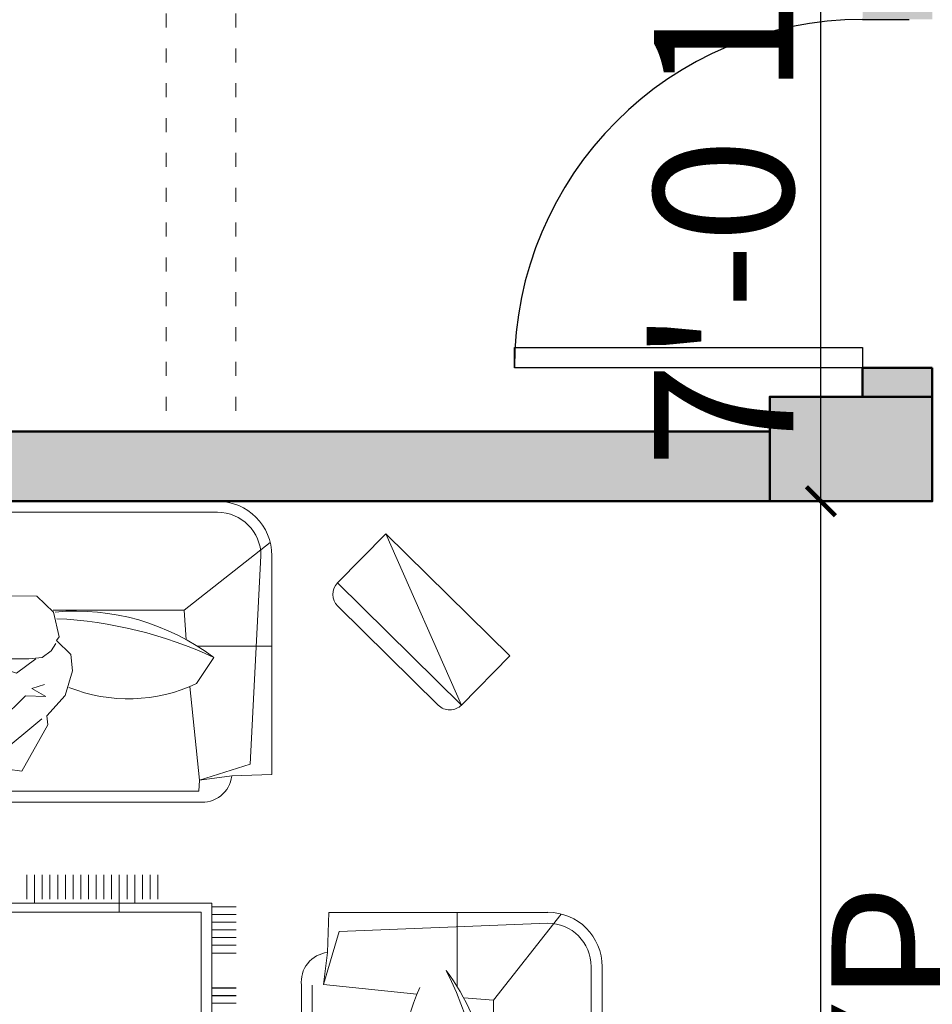
# Model space of a CAD drawing. Units: inches. Extents: x 375 to 1122, y 27 to 1069.
# Tile 76 of 155: x 588 to 667, y 792 to 877. Entities that reach past the tile are written whole.
import ezdxf

# ---------------------------------------------------------------- set-up
doc = ezdxf.new("R2010")
doc.units = ezdxf.units.IN
doc.linetypes.add('ACAD_ISO03W100', pattern=[30, 12, -18])
for name, color, linetype, lineweight in [('A-ANNO-DIMS', 2, 'Continuous', 18), ('A-COLS-PATT', 10, 'Continuous', 13), ('A-WALL-OVHD', 77, 'ACAD_ISO03W100', 18), ('A-WALL-PATT', 252, 'Continuous', 13), ('Columns', 10, 'Continuous', 50), ('Doors', 150, 'Continuous', 25), ('Furniture', 30, 'Continuous', 18), ('Walls', 250, 'Continuous', 50)]:
    doc.layers.add(name, color=color, linetype=linetype, lineweight=lineweight)
doc.styles.get("Standard").update_dxf_attribs({"font": 'arial.ttf'})
doc.dimstyles.new('ISO-25', dxfattribs={"dimtxt": 12, "dimasz": 2.5, "dimexe": 1.5, "dimexo": 1.5, "dimtad": 1, "dimdec": 1, "dimlunit": 3, "dimtxsty": 'Standard', "dimblk": 'ARCHTICK', "dimcen": 2.5, "dimadec": 0, "dimazin": 0, "dimtfac": 1, "dimtdec": 1, "dimtmove": 0, "dimatfit": 3, "dimfxl": 1.5, "dimfxlon": 1, "dimarcsym": 0})

# ---------------------------------------------------------------- blocks, each defined once
blk = doc.blocks.new('*U10')
for p, q in [((-30, 0), (-30, 4)), ((0, 0), (0, 4))]:
    blk.add_line(p, q)
blk.add_lwpolyline([(0, 0), (0, -30), (-1.75, -30), (-1.75, 0)], close=True)
blk.add_arc((0, 0), 30, 180, 270)
blk = doc.blocks.new('A$C4DC51D13')
for p, q in [((3265.3, 2996.2), (1188.4, 2996.2)), ((3265.3, 2962.7), (2590.4, 2962.7)), ((3778.5, 2897), (3631.2, 2747.3)), ((4008.9, 2375.5), (3778.5, 2897)), ((4156.2, 2525.2), (3778.5, 2897)), ((3163.3, 2664.8), (3425.7, 2870.9)), ((3397.7, 2830.3), (3364.5, 2194.8)), ((3430.8, 2163.8), (3430.8, 2830.3)), ((4008.9, 2375.5), (3631.2, 2747.3)), ((3631.7, 2676.6), (3938.2, 2375)), ((3163.3, 2664.8), (2764.7, 2664.8)), ((3170.4, 2574.2), (3163.3, 2664.8)), ((3430.8, 2554.4), (3204.1, 2554.4)), ((3253.7, 2520.5), (3201.8, 2440.8)), ((4008.9, 2375.5), (4156.2, 2525.2)), ((3210.5, 2146.7), (3181.5, 2431.8)), ((3364.5, 2194.8), (3210.5, 2146.7)), ((3308.6, 2159.3), (3430.8, 2163.8)), ((3208.9, 2113), (3210.5, 2146.7)), ((3308.6, 2159.3), (3210.5, 2146.7)), ((2614.2, 2113), (3208.9, 2113)), ((2614.2, 2079.9), (3208.9, 2079.9)), ((2684.5, 1784.3), (2684.5, 1858.2)), ((2708, 1772.3), (2708, 1858.2)), ((2731.5, 1784.3), (2731.5, 1858.2)), ((2754.9, 1784.3), (2754.9, 1858.2)), ((2778.4, 1784.3), (2778.4, 1858.2)), ((2801.9, 1784.3), (2801.9, 1858.2)), ((2825.4, 1784.3), (2825.4, 1858.2)), ((2848.8, 1784.3), (2848.8, 1858.2)), ((2872.3, 1784.3), (2872.3, 1858.2)), ((2895.8, 1784.3), (2895.8, 1858.2)), ((2919.3, 1784.3), (2919.3, 1858.2)), ((2942.7, 1784.3), (2942.7, 1858.2)), ((2966.2, 1744.8), (2966.2, 1858.2)), ((2989.7, 1784.3), (2989.7, 1858.2)), ((3013.2, 1772.3), (3013.2, 1858.2)), ((3036.6, 1784.3), (3036.6, 1858.2)), ((3060.1, 1784.3), (3060.1, 1858.2)), ((3083.6, 1784.3), (3083.6, 1858.2)), ((3248.4, 1772.3), (1158.5, 1772.3)), ((3248.4, 487.7), (3248.4, 1772.3)), ((1196, 1744.8), (3215.6, 1744.8)), ((3215.6, 511), (3215.6, 1744.8)), ((3248.8, 1760.8), (3322.7, 1760.8)), ((3600.6, 1621.7), (3605.1, 1743.8)), ((3605.1, 1743.8), (4271.6, 1743.8)), ((3995.7, 1743.8), (3995.7, 1517.1)), ((3248.8, 1737.3), (3322.7, 1737.3)), ((3248.8, 1713.8), (3322.7, 1713.8)), ((4271.6, 1710.7), (3636.1, 1685.8)), ((4106.1, 1476.4), (4312.2, 1738.8)), ((3248.8, 1690.4), (3322.7, 1690.4)), ((3636.1, 1685.8), (3588, 1523.6)), ((3248.8, 1666.9), (3322.7, 1666.9)), ((3248.8, 1643.4), (3322.7, 1643.4)), ((3248.8, 1619.9), (3322.7, 1619.9)), ((3600.6, 1621.7), (3588, 1523.6)), ((4404, 1578.3), (4404, 904.6)), ((4437.5, 165.9), (4437.5, 1578.3)), ((3248.8, 1513.8), (3322.7, 1513.8)), ((3248.8, 1513.3), (3322.7, 1513.3)), ((3521.2, 1130.7), (3521.2, 1521.9)), ((3554.3, 1131.4), (3554.3, 1521.9)), ((3588, 1523.6), (3873.1, 1494.5)), ((3248.8, 1490.4), (3322.7, 1490.4)), ((3248.8, 1489.9), (3322.7, 1489.9)), ((4015.5, 1483.4), (4106.1, 1476.4)), ((4106.1, 1476.4), (4106.1, 872.1)), ((3248.8, 1466.9), (3322.7, 1466.9))]:
    blk.add_line(p, q)
at = {"linetype": 'ByBlock'}
for points in [[(2625.9, 2180.3), (2669, 2174.2), (2748.1, 2315.4), (2745.8, 2342.6), (2801.2, 2404.9), (2823.9, 2479.6), (2818.4, 2529.9), (2775.1, 2571.7), (2782.4, 2583.3), (2765.2, 2658.8), (2714.5, 2706.9), (2634.6, 2708.6)], [(2563.4, 2654.7), (2512.2, 2609.3), (2506.2, 2548.3), (2540.1, 2504.4), (2576.9, 2490.9), (2579.8, 2539.3), (2598.7, 2543.6), (2636.7, 2516.4), (2690.3, 2516.7), (2731.2, 2520.1), (2758.5, 2540.1), (2773, 2563.3)], [(2712.3, 2515.8), (2652.7, 2472.4), (2603.2, 2489), (2580, 2503.6)], [(2738, 2438.2), (2699.2, 2425.4), (2742.4, 2401.4), (2680.4, 2403.2), (2604.1, 2328.3), (2519.2, 2273.3), (2529.8, 2261.8), (2402.7, 2252.7), (2395.4, 2241.1), (2431.1, 2241.3), (2375.7, 2196.9), (2385.2, 2181.2), (2474.4, 2199.5), (2549.9, 2234.6), (2596.2, 2223.2), (2730.1, 2333.1)]]:
    blk.add_lwpolyline(points, dxfattribs=at)
for centre, radius, start, end in [((3265.3, 2830.3), 165.9, 0, 90), ((3265.3, 2830.3), 132.4, 0, 90), ((3666.8, 2712.2), 50, 135.4503, 225.4503), ((2832.8, 1963.1), 698.5, 52.9389, 95.0789), ((2713.3, 1357.7), 1282.3, 65.0725, 87.2152), ((2993.8, 2882.7), 488.4, 248.2152, 295.2134), ((3973.2, 2410.6), 50, 225.4503, 315.4503), ((3219.2, 2169.3), 90, 263.4179, 353.5749), ((4271.6, 1578.3), 165.9, 0, 90), ((4271.6, 1578.3), 132.4, 0, 90), ((3610.6, 1532.2), 90, 96.4251, 186.5821), ((3383, 1136.2), 721.4, 348.1046, 36.6442), ((2968.3, 1058.8), 1115.8, 356.7543, 27.0804), ((4324, 1306.8), 488.4, 154.7866, 202.7137)]:
    blk.add_arc(centre, radius, start, end)
blk = doc.blocks.new('COLUMN-14X9IN')
blk.add_lwpolyline([(0, 0), (14, 0), (14, 9), (0, 9)], close=True)
blk = doc.blocks.new('_ArchTick')
at = {"color": 0, "linetype": 'ByBlock', "const_width": 0.15}
blk.add_lwpolyline([(-0.5, -0.5), (0.5, 0.5)], dxfattribs=at)
blk = doc.blocks.new('*D58')
at = {"layer": 'A-ANNO-DIMS', "color": 0, "lineweight": -2, "transparency": 16777216}
for p, q in [((656.912, 835.528), (656.912, 940.287)), ((655.412, 835.528), (658.412, 835.528)), ((656.912, 750.836), (656.912, 835.528)), ((655.412, 750.836), (658.412, 750.836))]:
    blk.add_line(p, q, dxfattribs=at)
at = {"layer": 'Defpoints', "color": 0, "transparency": 16777216}
for p in [(638.071, 835.528), (656.912, 835.528), (638.071, 750.836)]:
    blk.add_point(p, dxfattribs=at)
at = {"layer": 'A-ANNO-DIMS', "color": 0, "lineweight": -2, "transparency": 16777216, "xscale": 2.5, "yscale": 2.5, "zscale": 2.5}
for p, rotation in [((656.912, 835.528), 90), ((656.912, 750.836), 270)]:
    blk.add_blockref('_ArchTick', p, dxfattribs=dict(at, rotation=rotation))
at = {"layer": 'A-ANNO-DIMS', "color": 0, "transparency": 16777216, "insert": (650.082, 889.157), "char_height": 12, "attachment_point": 5, "rotation": 90}
blk.add_mtext('7\'-0 1/2" TYP.', dxfattribs=at)
blk = doc.blocks.new('*D79')
at = {"layer": 'A-ANNO-DIMS', "color": 0, "lineweight": -2, "transparency": 16777216}
for p, q in [((672.207, 647.528), (672.207, 810.92)), ((670.707, 647.528), (673.707, 647.528)), ((672.207, 589.528), (672.207, 647.528)), ((670.707, 589.528), (673.707, 589.528))]:
    blk.add_line(p, q, dxfattribs=at)
at = {"layer": 'Defpoints', "color": 0, "transparency": 16777216}
for p in [(663.507, 647.528), (672.207, 647.528), (663.507, 589.528)]:
    blk.add_point(p, dxfattribs=at)
at = {"layer": 'A-ANNO-DIMS', "color": 0, "lineweight": -2, "transparency": 16777216, "xscale": 2.5, "yscale": 2.5, "zscale": 2.5}
for p, rotation in [((672.207, 647.528), 90), ((672.207, 589.528), 270)]:
    blk.add_blockref('_ArchTick', p, dxfattribs=dict(at, rotation=rotation))
at = {"layer": 'A-ANNO-DIMS', "color": 0, "transparency": 16777216, "insert": (665.378, 730.474), "char_height": 12, "attachment_point": 5, "rotation": 90}
blk.add_mtext('CABINET 4\'-10" TYP.', dxfattribs=at)
blk = doc.blocks.new('*D82')
at = {"layer": 'A-ANNO-DIMS', "color": 0, "lineweight": -2, "transparency": 16777216}
for p, q in [((401.507, 1009.528), (398.507, 1009.528)), ((400.007, 160.528), (400.007, 1009.528)), ((401.507, 160.528), (398.507, 160.528))]:
    blk.add_line(p, q, dxfattribs=at)
at = {"layer": 'Defpoints', "color": 0, "transparency": 16777216}
for p in [(400.007, 1009.528), (630.534, 1009.528), (630.534, 160.528)]:
    blk.add_point(p, dxfattribs=at)
at = {"layer": 'A-ANNO-DIMS', "color": 0, "lineweight": -2, "transparency": 16777216, "xscale": 2.5, "yscale": 2.5, "zscale": 2.5}
for p, rotation in [((400.007, 1009.528), 90), ((400.007, 160.528), 270)]:
    blk.add_blockref('_ArchTick', p, dxfattribs=dict(at, rotation=rotation))
at = {"layer": 'A-ANNO-DIMS', "color": 0, "transparency": 16777216, "insert": (393.255, 585.028), "char_height": 12, "attachment_point": 5, "rotation": 90}
blk.add_mtext('70\'-9"', dxfattribs=at)
blk = doc.blocks.new('*D85')
at = {"layer": 'A-ANNO-DIMS', "color": 0, "lineweight": -2, "transparency": 16777216}
for p, q in [((401.507, 868.528), (398.507, 868.528)), ((400.007, 814.528), (400.007, 868.528)), ((401.507, 814.528), (398.507, 814.528))]:
    blk.add_line(p, q, dxfattribs=at)
at = {"layer": 'Defpoints', "color": 0, "transparency": 16777216}
for p in [(400.007, 868.528), (845.007, 868.528), (845.007, 814.528)]:
    blk.add_point(p, dxfattribs=at)
at = {"layer": 'A-ANNO-DIMS', "color": 0, "lineweight": -2, "transparency": 16777216, "xscale": 2.5, "yscale": 2.5, "zscale": 2.5}
for p, rotation in [((400.007, 868.528), 90), ((400.007, 814.528), 270)]:
    blk.add_blockref('_ArchTick', p, dxfattribs=dict(at, rotation=rotation))
at = {"layer": 'A-ANNO-DIMS', "color": 0, "transparency": 16777216, "insert": (393.255, 841.528), "char_height": 12, "attachment_point": 5, "rotation": 90}
blk.add_mtext('4\'-6"', dxfattribs=at)
blk = doc.blocks.new('*D92')
at = {"layer": 'A-ANNO-DIMS', "color": 0, "lineweight": -2, "transparency": 16777216}
for p, q in [((621.507, 1052.528), (621.507, 1055.528)), ((657.507, 1052.528), (657.507, 1055.528)), ((621.507, 1054.028), (657.507, 1054.028))]:
    blk.add_line(p, q, dxfattribs=at)
at = {"layer": 'Defpoints', "color": 0, "transparency": 16777216}
for p in [(657.507, 1054.028), (621.507, 460.528), (657.507, 460.528)]:
    blk.add_point(p, dxfattribs=at)
at = {"layer": 'A-ANNO-DIMS', "color": 0, "lineweight": -2, "transparency": 16777216, "xscale": 2.5, "yscale": 2.5, "zscale": 2.5, "rotation": 180}
blk.add_blockref('_ArchTick', (621.507, 1054.028), dxfattribs=at)
at = {"layer": 'A-ANNO-DIMS', "color": 0, "lineweight": -2, "transparency": 16777216, "xscale": 2.5, "yscale": 2.5, "zscale": 2.5}
blk.add_blockref('_ArchTick', (657.507, 1054.028), dxfattribs=at)
at = {"layer": 'A-ANNO-DIMS', "color": 0, "transparency": 16777216, "insert": (639.507, 1060.784), "char_height": 12, "attachment_point": 5}
blk.add_mtext('3\'-0"', dxfattribs=at)

msp = doc.modelspace()

# ---------------------------------------------------------------- hatches: boundary and pattern name
at = {"layer": 'A-COLS-PATT'}
h = msp.add_hatch(color=256, dxfattribs=at)
h.dxf.hatch_style = 1
h.paths.add_polyline_path([(512.507, 982.528), (498.507, 982.528), (498.507, 973.528), (512.507, 973.528)])
h.paths.add_polyline_path([(666.507, 982.528), (652.507, 982.528), (652.507, 973.528), (666.507, 973.528)])
h.paths.add_polyline_path([(802.007, 982.528), (788.007, 982.528), (788.007, 973.528), (802.007, 973.528)])
h.paths.add_polyline_path([(932.007, 982.528), (918.007, 982.528), (918.007, 973.528), (932.007, 973.528)])
h.paths.add_polyline_path([(507.507, 841.528), (498.507, 841.528), (498.507, 827.528), (507.507, 827.528)])
h.paths.add_polyline_path([(666.507, 844.528), (652.507, 844.528), (652.507, 835.528), (666.507, 835.528)])
h.paths.add_polyline_path([(802.007, 814.528), (788.007, 814.528), (788.007, 805.528), (802.007, 805.528)])
h.paths.add_polyline_path([(932.007, 814.528), (918.007, 814.528), (918.007, 805.528), (932.007, 805.528)])
h.paths.add_polyline_path([(507.507, 719.528), (498.507, 719.528), (498.507, 705.528), (507.507, 705.528)])
h.paths.add_polyline_path([(731.007, 676.528), (722.007, 676.528), (722.007, 662.528), (731.007, 662.528)])
h.paths.add_polyline_path([(802.007, 676.528), (788.007, 676.528), (788.007, 667.528), (802.007, 667.528)])
h.paths.add_polyline_path([(932.007, 676.528), (918.007, 676.528), (918.007, 667.528), (932.007, 667.528)])
h.paths.add_polyline_path([(932.007, 583.528), (918.007, 583.528), (918.007, 574.528), (932.007, 574.528)])
h.paths.add_polyline_path([(868.007, 583.528), (854.007, 583.528), (854.007, 574.528), (868.007, 574.528)])
h.paths.add_polyline_path([(868.007, 502.528), (854.007, 502.528), (854.007, 493.528), (868.007, 493.528)])
h.paths.add_polyline_path([(932.007, 502.528), (918.007, 502.528), (918.007, 493.528), (932.007, 493.528)])
h.paths.add_polyline_path([(672.507, 592.028), (663.507, 592.028), (663.507, 578.028), (672.507, 578.028)])
h.paths.add_polyline_path([(512.507, 589.528), (498.507, 589.528), (498.507, 580.528), (512.507, 580.528)])
h.paths.add_polyline_path([(507.507, 464.528), (498.507, 464.528), (498.507, 450.528), (507.507, 450.528)])
h.paths.add_polyline_path([(731.007, 507.528), (722.007, 507.528), (722.007, 493.528), (731.007, 493.528)])
h.paths.add_polyline_path([(802.007, 502.528), (788.007, 502.528), (788.007, 493.528), (802.007, 493.528)])
h.paths.add_polyline_path([(507.507, 342.528), (498.507, 342.528), (498.507, 328.528), (507.507, 328.528)])
h.paths.add_polyline_path([(512.507, 196.528), (498.507, 196.528), (498.507, 187.528), (512.507, 187.528)])
h.paths.add_polyline_path([(666.507, 334.528), (652.507, 334.528), (652.507, 325.528), (666.507, 325.528)])
h.paths.add_polyline_path([(666.507, 196.528), (652.507, 196.528), (652.507, 187.528), (666.507, 187.528)])
h.paths.add_polyline_path([(805.007, 196.528), (791.007, 196.528), (791.007, 187.528), (805.007, 187.528)])
h.paths.add_polyline_path([(932.007, 196.528), (918.007, 196.528), (918.007, 187.528), (932.007, 187.528)])
h.paths.add_polyline_path([(932.007, 334.528), (918.007, 334.528), (918.007, 325.528), (932.007, 325.528)])
h.paths.add_polyline_path([(805.007, 334.528), (791.007, 334.528), (791.007, 325.528), (805.007, 325.528)])
at = {"layer": 'A-WALL-PATT'}
h = msp.add_hatch(color=256, dxfattribs=at)
h.dxf.hatch_style = 1
h.paths.add_polyline_path([(962.007, 388.528), (989.007, 388.528), (989.007, 394.528), (962.007, 394.528), (932.007, 394.528), (932.007, 397.528), (923.007, 397.528), (923.007, 394.528), (842.007, 394.528), (842.007, 334.528), (839.507, 334.528), (839.507, 328.528), (854.007, 328.528), (854.007, 334.528), (848.007, 334.528), (848.007, 388.528), (953.007, 388.528), (953.007, 356.081), (962.007, 356.081), (962.007, 358.554), (989.007, 358.554), (989.007, 364.554), (962.007, 364.554)])
h.paths.add_polyline_path([(989.007, 502.528), (932.007, 502.528), (932.007, 583.528), (932.007, 593.528), (923.007, 593.528), (923.007, 583.528), (854.007, 583.528), (854.007, 556.528), (863.007, 556.528), (863.007, 574.528), (923.007, 574.528), (923.007, 502.528), (863.007, 502.528), (863.007, 520.528), (854.007, 520.528), (854.007, 502.528), (773.007, 502.528), (773.007, 493.528), (788.007, 493.528), (788.007, 402.028), (722.007, 402.028), (722.007, 373.528), (728.007, 373.528), (728.007, 396.028), (788.007, 396.028), (788.007, 373.528), (794.007, 373.528), (794.007, 430.528), (814.007, 430.528), (814.007, 436.528), (794.007, 436.528), (794.007, 493.528), (923.007, 493.528), (923.007, 487.528), (932.007, 487.528), (932.007, 493.528), (983.007, 493.528), (983.007, 473.528), (989.007, 473.528)])
h.paths.add_polyline_path([(797.007, 325.528), (805.007, 325.528), (805.007, 328.528), (807.507, 328.528), (807.507, 334.528), (791.007, 334.528), (791.007, 226.528), (770.757, 226.528), (770.757, 217.528), (791.007, 217.528), (791.007, 187.528), (855.007, 187.528), (855.007, 196.528), (797.007, 196.528)])
h.paths.add_polyline_path([(989.007, 238.528), (962.007, 238.528), (962.007, 256.424), (953.007, 256.424), (953.007, 229.528), (980.007, 229.528), (980.007, 196.528), (915.007, 196.528), (915.007, 187.528), (989.007, 187.528)])
h.paths.add_polyline_path([(962.007, 334.528), (884.007, 334.528), (884.007, 328.528), (918.007, 328.528), (918.007, 325.528), (932.007, 325.528), (932.007, 328.528), (953.007, 328.528), (953.007, 304.424), (962.007, 304.424)])
h.paths.add_polyline_path([(606.507, 283.528), (609.507, 283.528), (609.507, 289.528), (600.507, 289.528), (600.507, 196.528), (578.507, 196.528), (578.507, 187.528), (606.507, 187.528), (606.507, 196.528)])
h.paths.add_polyline_path([(666.507, 292.528), (660.507, 292.528), (660.507, 289.528), (633.507, 289.528), (633.507, 283.528), (660.507, 283.528), (660.507, 196.528), (628.007, 196.528), (628.007, 187.528), (630.534, 187.528), (630.534, 160.528), (636.534, 160.528), (636.534, 187.528), (660.507, 187.528), (660.507, 160.528), (666.507, 160.528), (666.507, 217.528), (686.757, 217.528), (686.757, 226.528), (666.507, 226.528)])
h.paths.add_polyline_path([(480.507, 256.424), (471.507, 256.424), (471.507, 238.528), (444.507, 238.528), (444.507, 187.528), (518.507, 187.528), (518.507, 196.528), (453.507, 196.528), (453.507, 229.528), (480.507, 229.528)])
h.paths.add_polyline_path([(480.507, 328.528), (652.507, 328.528), (652.507, 325.528), (660.507, 325.528), (660.507, 322.528), (666.507, 322.528), (666.507, 334.528), (507.507, 334.528), (507.507, 360.528), (498.507, 360.528), (498.507, 334.528), (471.507, 334.528), (471.507, 304.424), (480.507, 304.424)])
h.paths.add_polyline_path([(507.507, 484.528), (498.507, 484.528), (498.507, 444.528), (507.507, 444.528), (507.507, 454.528), (621.507, 454.528), (621.507, 460.528), (507.507, 460.528)])
h.paths.add_polyline_path([(672.507, 604.528), (683.257, 604.528), (683.257, 613.528), (669.507, 613.528), (669.507, 649.528), (663.507, 649.528), (663.507, 589.528), (507.507, 589.528), (507.507, 613.528), (498.507, 613.528), (498.507, 556.528), (507.507, 556.528), (507.507, 580.528), (663.507, 580.528), (663.507, 520.528), (669.507, 520.528), (669.507, 556.528), (683.257, 556.528), (683.257, 565.528), (672.507, 565.528)])
h.paths.add_polyline_path([(731.007, 667.528), (734.007, 667.528), (734.007, 676.528), (728.007, 676.528), (728.007, 715.528), (657.507, 715.528), (657.507, 709.528), (663.507, 709.528), (663.507, 673.528), (669.507, 673.528), (669.507, 709.528), (722.007, 709.528), (722.007, 613.528), (704.757, 613.528), (704.757, 604.528), (722.007, 604.528), (722.007, 565.528), (704.757, 565.528), (704.757, 556.528), (722.007, 556.528), (722.007, 502.528), (722.007, 460.528), (669.507, 460.528), (669.507, 496.528), (663.507, 496.528), (663.507, 460.528), (657.507, 460.528), (657.507, 454.528), (728.007, 454.528), (728.007, 493.528), (734.007, 493.528), (734.007, 502.528), (731.007, 502.528)])
h.paths.add_polyline_path([(986.007, 718.528), (959.007, 718.528), (959.007, 727.528), (950.007, 727.528), (950.007, 709.528), (977.007, 709.528), (977.007, 676.528), (794.007, 676.528), (794.007, 805.528), (802.007, 805.528), (802.007, 808.528), (804.507, 808.528), (804.507, 814.528), (788.007, 814.528), (788.007, 774.028), (728.007, 774.028), (728.007, 796.528), (722.007, 796.528), (722.007, 768.028), (788.007, 768.028), (788.007, 676.528), (773.007, 676.528), (773.007, 667.528), (923.007, 667.528), (923.007, 657.528), (932.007, 657.528), (932.007, 667.528), (986.007, 667.528)])
h.paths.add_polyline_path([(621.507, 715.528), (507.507, 715.528), (507.507, 733.528), (498.507, 733.528), (498.507, 715.528), (498.507, 685.528), (507.507, 685.528), (507.507, 709.528), (621.507, 709.528)])
h.paths.add_polyline_path([(666.507, 847.028), (660.507, 847.028), (660.507, 844.528), (652.507, 844.528), (652.507, 841.528), (480.507, 841.528), (480.507, 859.528), (471.507, 859.528), (471.507, 835.528), (498.507, 835.528), (498.507, 817.528), (507.507, 817.528), (507.507, 835.528), (666.507, 835.528)])
h.paths.add_polyline_path([(480.507, 940.528), (453.507, 940.528), (453.507, 973.528), (518.507, 973.528), (518.507, 982.528), (444.507, 982.528), (444.507, 931.528), (471.507, 931.528), (471.507, 907.528), (480.507, 907.528)])
h.paths.add_polyline_path([(606.507, 982.528), (578.507, 982.528), (578.507, 973.528), (600.507, 973.528), (600.507, 880.528), (609.507, 880.528), (609.507, 886.528), (606.507, 886.528)])
h.paths.add_polyline_path([(666.507, 943.528), (686.757, 943.528), (686.757, 952.528), (666.507, 952.528), (666.507, 1009.528), (660.507, 1009.528), (660.507, 982.528), (636.534, 982.528), (636.534, 1009.528), (630.534, 1009.528), (630.534, 982.528), (628.007, 982.528), (628.007, 973.528), (660.507, 973.528), (660.507, 886.528), (633.507, 886.528), (633.507, 880.528), (660.507, 880.528), (660.507, 877.028), (666.507, 877.028)])
h.paths.add_polyline_path([(986.007, 874.528), (932.007, 874.528), (932.007, 877.528), (923.007, 877.528), (923.007, 874.528), (788.007, 874.528), (788.007, 868.528), (788.007, 844.528), (794.007, 844.528), (794.007, 868.528), (839.007, 868.528), (839.007, 814.528), (836.507, 814.528), (836.507, 808.528), (851.007, 808.528), (851.007, 814.528), (845.007, 814.528), (845.007, 868.528), (986.007, 868.528)])
h.paths.add_polyline_path([(959.007, 838.554), (986.007, 838.554), (986.007, 844.554), (959.007, 844.554), (959.007, 847.028), (950.007, 847.028), (950.007, 814.528), (881.007, 814.528), (881.007, 808.528), (918.007, 808.528), (918.007, 805.528), (932.007, 805.528), (932.007, 808.528), (950.007, 808.528), (950.007, 793.528), (959.007, 793.528)])
h.paths.add_polyline_path([(986.007, 982.528), (899.007, 982.528), (899.007, 973.528), (923.007, 973.528), (923.007, 967.528), (932.007, 967.528), (932.007, 973.528), (980.007, 973.528), (980.007, 953.528), (986.007, 953.528)])
h.paths.add_polyline_path([(851.007, 982.528), (788.007, 982.528), (788.007, 952.528), (770.757, 952.528), (770.757, 943.528), (788.007, 943.528), (788.007, 910.528), (814.007, 910.528), (814.007, 916.528), (794.007, 916.528), (794.007, 973.528), (851.007, 973.528)])

# ---------------------------------------------------------------- linework, layer by layer
at = {"layer": 'A-WALL-OVHD', "ltscale": 0.1}
for p, q in [((600.507, 880.528), (600.507, 841.528)), ((606.507, 880.528), (606.507, 841.528))]:
    msp.add_line(p, q, dxfattribs=at)
at = {"layer": 'Walls'}
for p, q in [((660.507, 844.528), (660.507, 847.028)), ((660.507, 847.028), (666.507, 847.028)), ((666.507, 835.528), (666.507, 847.028)), ((652.507, 841.528), (652.507, 844.528)), ((652.507, 844.528), (660.507, 844.528)), ((480.507, 841.528), (652.507, 841.528)), ((507.507, 835.528), (666.507, 835.528))]:
    msp.add_line(p, q, dxfattribs=at)

# ---------------------------------------------------------------- block references
at = {"layer": 'Columns'}
msp.add_blockref('COLUMN-14X9IN', (652.507, 835.528), dxfattribs=at)
at = {"layer": 'Doors', "rotation": 270}
msp.add_blockref('*U10', (660.507, 847.028), dxfattribs=at)
at = {"layer": 'Furniture', "xscale": 0.0282665567793757, "yscale": 0.0282665567793757, "zscale": 0.0282665567793757}
msp.add_blockref('A$C4DC51D13', (512.638, 750.836), dxfattribs=at)

# ---------------------------------------------------------------- dimensions: what is measured, and where the dimension line sits
at = {"layer": 'A-ANNO-DIMS'}
dim = msp.add_linear_dim(base=(657.507, 1054.028), p1=(621.507, 460.528), p2=(657.507, 460.528), dimstyle='ISO-25', override={"dimdec": 1, "dimlfac": 1, "dimrnd": 0, "dimzin": 1, "dimdsep": 46, "dimlunit": 4, "dimfrac": 2}, dxfattribs=at)
dim.commit()
dim.dimension.update_dxf_attribs({"geometry": '*D92', "text_midpoint": (639.507, 1060.784)})
for base, p1, p2, picture, middle in [((400.007, 1009.528), (630.534, 160.528), (630.534, 1009.528), '*D82', (393.255, 585.028)), ((400.007, 868.528), (845.007, 814.528), (845.007, 868.528), '*D85', (393.255, 841.528))]:
    dim = msp.add_linear_dim(base=base, p1=p1, p2=p2, angle=90, dimstyle='ISO-25', override={"dimdec": 1, "dimlfac": 1, "dimrnd": 0, "dimzin": 1, "dimdsep": 46, "dimlunit": 4, "dimfrac": 2}, dxfattribs=at)
    dim.commit()
    dim.dimension.update_dxf_attribs({"geometry": picture, "text_midpoint": middle})
for base, p1, p2, text, picture, middle in [((656.912, 835.528), (638.071, 750.836), (638.071, 835.528), '<> TYP.', '*D58', (650.082, 889.157)), ((672.207, 647.528), (663.507, 589.528), (663.507, 647.528), 'CABINET <> TYP.', '*D79', (665.378, 730.474))]:
    dim = msp.add_linear_dim(base=base, p1=p1, p2=p2, angle=90, text=text, dimstyle='ISO-25', override={"dimdec": 1, "dimlfac": 1, "dimrnd": 0, "dimzin": 1, "dimdsep": 46, "dimlunit": 4, "dimfrac": 2}, dxfattribs=at)
    dim.commit()
    dim.dimension.update_dxf_attribs({"geometry": picture, "text_midpoint": middle})

doc.saveas('drawing.dxf')
